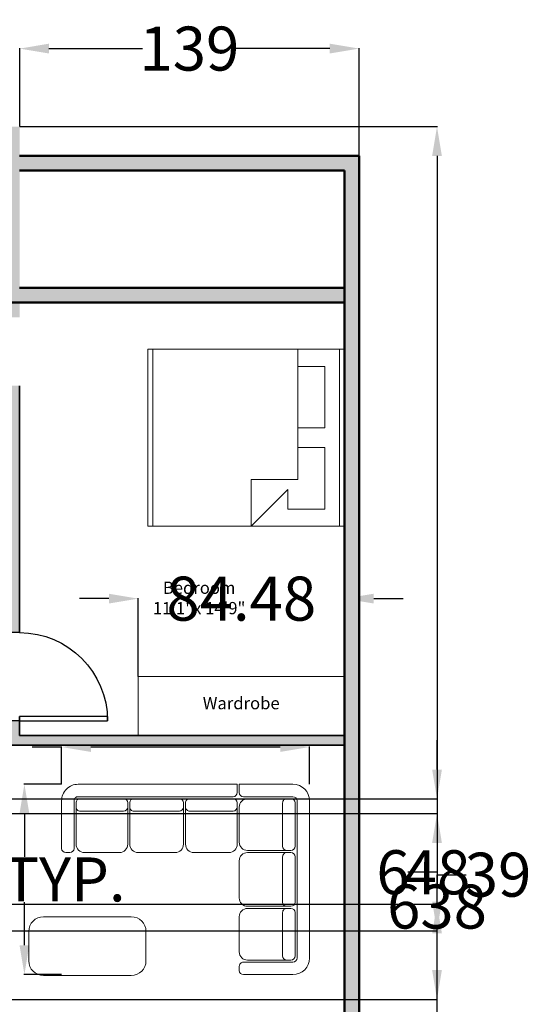
# Model space of a CAD drawing. Units: inches. Extents: x 2 to 695, y -374 to 352.
# Tile 6 of 6: x 421 to 630, y -51 to 352. Entities that reach past the tile are written whole.
import ezdxf

# ---------------------------------------------------------------- set-up
doc = ezdxf.new("R2010")
doc.units = ezdxf.units.IN
for name, color, linetype, lineweight in [('A-ANNO-DIMS', 2, 'Continuous', 18), ('A-ANNO-TEXT', 7, 'Continuous', 18), ('A-AREA-IDEN', 7, 'Continuous', 18), ('A-DOOR', 3, 'Continuous', 25), ('A-WALL-PATT', 252, 'Continuous', 13), ('Furniture', 2, 'Continuous', 18), ('Inner Wall', 5, 'Continuous', 35), ('Outer Wall', 1, 'Continuous', 50)]:
    doc.layers.add(name, color=color, linetype=linetype, lineweight=lineweight)
doc.styles.get("Standard").update_dxf_attribs({"font": 'arial.ttf'})
doc.dimstyles.get("Standard").update_dxf_attribs({"dimtxt": 18, "dimasz": 12, "dimexe": 0.18, "dimexo": 0.0625, "dimgap": 0.09, "dimtad": 0, "dimtih": 1, "dimtoh": 1, "dimdec": 0, "dimzin": 0, "dimdsep": 46, "dimlunit": 3, "dimtxsty": 'Standard', "dimcen": 0.09, "dimadec": 0, "dimazin": 0, "dimtfac": 1, "dimtdec": 0, "dimtofl": 0, "dimtmove": 0, "dimatfit": 3, "dimfxl": 1, "dimtolj": 1, "dimtzin": 0, "dimarcsym": 0})

# ---------------------------------------------------------------- blocks, each defined once
blk = doc.blocks.new('*U2')
for p, q in [((0, 0), (0, -4)), ((36, 0), (36, -4))]:
    blk.add_line(p, q)
blk.add_lwpolyline([(0, 0), (0, 36), (1.75, 36), (1.75, 0)], close=True)
blk.add_arc((0, 0), 36, 0, 90)
blk = doc.blocks.new('A$C2AFA021D')
for p, q in [((0.8, 2.3), (0.2, 2.3)), ((0.2, 2.15), (0.8, 2.15)), ((0.85, 2.2), (0.85, 2.25)), ((0, 2.1), (0, 0.2)), ((0.15, 0.2), (0.15, 2.1)), ((0.175, 1.55), (0.175, 2.075)), ((0.225, 2.125), (0.275, 2.125)), ((0.75, 2.125), (0.275, 2.125)), ((0.325, 2.075), (0.325, 1.55)), ((0.85, 1.6), (0.85, 2.025)), ((0.275, 1.5), (0.225, 1.5)), ((0.225, 1.475), (0.275, 1.475)), ((0.275, 1.5), (0.75, 1.5)), ((0.75, 1.475), (0.275, 1.475)), ((0.175, 0.875), (0.175, 1.425)), ((0.325, 1.425), (0.325, 0.875)), ((0.85, 0.925), (0.85, 1.375)), ((0.175, 0.225), (0.175, 0.75)), ((0.275, 0.825), (0.225, 0.825)), ((0.225, 0.8), (0.275, 0.8)), ((0.275, 0.825), (0.75, 0.825)), ((0.75, 0.8), (0.275, 0.8)), ((0.325, 0.75), (0.325, 0.225)), ((0.875, 0.275), (0.875, 0.725)), ((0.975, 0.825), (1.4, 0.825)), ((1.5, 0.725), (1.5, 0.275)), ((1.525, 0.275), (1.525, 0.725)), ((1.625, 0.825), (2.075, 0.825)), ((2.175, 0.725), (2.175, 0.275)), ((2.2, 0.275), (2.2, 0.725)), ((2.3, 0.825), (2.725, 0.825)), ((2.825, 0.725), (2.825, 0.275)), ((2.85, 0.2), (2.85, 0.775)), ((2.9, 0.825), (2.95, 0.825)), ((3, 0.775), (3, 0.2)), ((0.85, 0.275), (0.85, 0.7)), ((0.875, 0.275), (0.875, 0.225)), ((1.45, 0.325), (0.925, 0.325)), ((1.5, 0.225), (1.5, 0.275)), ((1.525, 0.275), (1.525, 0.225)), ((2.125, 0.325), (1.575, 0.325)), ((2.175, 0.225), (2.175, 0.275)), ((2.2, 0.275), (2.2, 0.225)), ((2.775, 0.325), (2.25, 0.325)), ((2.825, 0.225), (2.825, 0.275)), ((0.8, 0.15), (0.2, 0.15)), ((0.275, 0.175), (0.225, 0.175)), ((0.275, 0.175), (0.75, 0.175)), ((0.925, 0.175), (1.45, 0.175)), ((0.925, 0.15), (2.8, 0.15)), ((1.575, 0.175), (2.125, 0.175)), ((2.25, 0.175), (2.775, 0.175)), ((0.85, 0), (0.85, 0.1)), ((0.875, 0.1), (0.875, 0)), ((0.2, 0), (0.85, 0)), ((2.8, 0), (0.875, 0))]:
    blk.add_line(p, q)
for centre, radius, start, end in [((0.2, 2.1), 0.2, 90, 180), ((0.8, 2.25), 0.05, 0, 90), ((0.2, 2.1), 0.05, 90, 180), ((0.8, 2.2), 0.05, 270, 0), ((0.225, 2.075), 0.05, 90, 180), ((0.275, 2.075), 0.05, 0, 90), ((0.75, 2.025), 0.1, 0, 90), ((0.225, 1.55), 0.05, 180, 270), ((0.275, 1.55), 0.05, 270, 0), ((0.75, 1.6), 0.1, 270, 0), ((0.225, 1.425), 0.05, 90, 180), ((0.275, 1.425), 0.05, 0, 90), ((0.75, 1.375), 0.1, 360, 90), ((0.225, 0.875), 0.05, 180, 270), ((0.275, 0.875), 0.05, 270, 0), ((0.75, 0.925), 0.1, 270, 0), ((0.225, 0.75), 0.05, 90, 180), ((0.275, 0.75), 0.05, 0, 90), ((0.75, 0.7), 0.1, 0, 90), ((0.975, 0.725), 0.1, 90, 180), ((1.4, 0.725), 0.1, 0, 90), ((1.625, 0.725), 0.1, 90, 180), ((2.075, 0.725), 0.1, 0, 90), ((2.3, 0.725), 0.1, 90, 180), ((2.725, 0.725), 0.1, 0, 90), ((2.9, 0.775), 0.05, 90, 180), ((2.95, 0.775), 0.05, 0, 90), ((0.75, 0.275), 0.1, 270, 0), ((0.925, 0.275), 0.05, 90, 180), ((1.45, 0.275), 0.05, 360, 90), ((1.575, 0.275), 0.05, 90, 180), ((2.125, 0.275), 0.05, 360, 90), ((2.25, 0.275), 0.05, 90, 180), ((2.775, 0.275), 0.05, 360, 90), ((0.2, 0.2), 0.2, 180, 270), ((0.2, 0.2), 0.05, 180, 270), ((0.225, 0.225), 0.05, 180, 270), ((0.275, 0.225), 0.05, 270, 0), ((0.8, 0.1), 0.05, 0, 90), ((0.925, 0.225), 0.05, 180, 270), ((0.925, 0.1), 0.05, 90, 180), ((1.45, 0.225), 0.05, 270, 0), ((1.575, 0.225), 0.05, 180, 270), ((2.125, 0.225), 0.05, 270, 0), ((2.25, 0.225), 0.05, 180, 270), ((2.775, 0.225), 0.05, 270, 0), ((2.8, 0.2), 0.2, 270, 0), ((2.8, 0.2), 0.05, 270, 0)]:
    blk.add_arc(centre, radius, start, end)
blk = doc.blocks.new('KING-00')
for p, q in [((-0.897, -0.947), (-0.897, 0.882)), ((0.602, 0.882), (0.602, -0.464)), ((1.034, -0.947), (1.034, 0.882)), ((0.602, 0.704), (0.881, 0.704)), ((0.881, 0.069), (0.881, 0.704)), ((0.602, 0.069), (0.881, 0.069)), ((0.881, -0.134), (0.602, -0.134)), ((0.881, -0.769), (0.881, -0.134)), ((0.119, -0.464), (0.119, -0.947)), ((0.602, -0.464), (0.119, -0.464)), ((0.119, -0.947), (0.5, -0.566)), ((0.5, -0.769), (0.5, -0.566)), ((0.5, -0.769), (0.881, -0.769))]:
    blk.add_line(p, q)
blk.add_lwpolyline([(-0.948, -0.947), (-0.948, 0.882), (1.084, 0.882), (1.084, -0.947)], close=True)
blk = doc.blocks.new('*D18')
at = {"layer": 'A-ANNO-DIMS', "color": 0, "lineweight": -2, "transparency": 16777216}
for p, q in [((437.96, 54.39), (425.96, 54.39)), ((437.96, 39.23), (437.96, 54.57)), ((527.48, 54.39), (449.96, 54.39)), ((539.48, 39.23), (539.48, 54.57))]:
    blk.add_line(p, q, dxfattribs=at)
at = {"layer": 'A-ANNO-DIMS', "color": 0, "transparency": 16777216}
for points in [[(449.96, 56.39), (449.96, 52.39), (437.96, 54.39)], [(527.48, 56.39), (527.48, 52.39), (539.48, 54.39)]]:
    blk.add_solid(points, dxfattribs=at)
at = {"layer": 'Defpoints', "color": 0, "transparency": 16777216}
for p in [(437.96, 54.39), (437.96, 39.17), (539.48, 39.17)]:
    blk.add_point(p, dxfattribs=at)
at = {"layer": 'A-ANNO-DIMS', "color": 0, "transparency": 16777216, "insert": (337.39, 54.39), "char_height": 18, "attachment_point": 5}
blk.add_mtext('\\A1;SOFA 102 TYP.', dxfattribs=at)
blk = doc.blocks.new('*D19')
at = {"layer": 'A-ANNO-DIMS', "color": 0, "lineweight": -2, "transparency": 16777216}
for p, q in [((437.9, 39.17), (422.55, 39.17)), ((422.73, 27.17), (422.73, 9.53)), ((422.73, -26.67), (422.73, -9.03)), ((437.9, -38.67), (422.55, -38.67))]:
    blk.add_line(p, q, dxfattribs=at)
at = {"layer": 'A-ANNO-DIMS', "color": 0, "transparency": 16777216}
for points in [[(420.73, 27.17), (424.73, 27.17), (422.73, 39.17)], [(420.73, -26.67), (424.73, -26.67), (422.73, -38.67)]]:
    blk.add_solid(points, dxfattribs=at)
at = {"layer": 'Defpoints', "color": 0, "transparency": 16777216}
for p in [(437.96, 39.17), (422.73, -38.67), (437.96, -38.67)]:
    blk.add_point(p, dxfattribs=at)
at = {"layer": 'A-ANNO-DIMS', "color": 0, "transparency": 16777216, "insert": (422.73, 0.25), "char_height": 18, "attachment_point": 5}
blk.add_mtext('\\A1;78 TYP.', dxfattribs=at)
blk = doc.blocks.new('*D29')
at = {"layer": 'A-ANNO-DIMS', "color": 0, "lineweight": -2, "transparency": 16777216}
for p, q in [((420.85, 308.13), (591.88, 308.13)), ((591.7, 296.13), (591.7, -1.56)), ((591.7, -317.82), (591.7, -20.13)), ((217.35, -329.82), (591.88, -329.82))]:
    blk.add_line(p, q, dxfattribs=at)
at = {"layer": 'A-ANNO-DIMS', "color": 0, "transparency": 16777216}
for points in [[(589.7, 296.13), (593.7, 296.13), (591.7, 308.13)], [(589.7, -317.82), (593.7, -317.82), (591.7, -329.82)]]:
    blk.add_solid(points, dxfattribs=at)
at = {"layer": 'Defpoints', "color": 0, "transparency": 16777216}
for p in [(420.79, 308.13), (591.7, 308.13), (217.29, -329.82)]:
    blk.add_point(p, dxfattribs=at)
at = {"layer": 'A-ANNO-DIMS', "color": 0, "transparency": 16777216, "insert": (591.7, -10.85), "char_height": 18, "attachment_point": 5}
blk.add_mtext('\\A1;638', dxfattribs=at)
blk = doc.blocks.new('*D32')
at = {"layer": 'A-ANNO-DIMS', "color": 0, "lineweight": -2, "transparency": 16777216}
for p, q in [((420.79, 308.19), (420.79, 340.22)), ((432.79, 340.04), (471.14, 340.04)), ((547.79, 340.04), (509.43, 340.04)), ((559.79, 296.24), (559.79, 340.22))]:
    blk.add_line(p, q, dxfattribs=at)
at = {"layer": 'A-ANNO-DIMS', "color": 0, "transparency": 16777216}
for points in [[(432.79, 342.04), (432.79, 338.04), (420.79, 340.04)], [(547.79, 342.04), (547.79, 338.04), (559.79, 340.04)]]:
    blk.add_solid(points, dxfattribs=at)
at = {"layer": 'Defpoints', "color": 0, "transparency": 16777216}
for p in [(559.79, 340.04), (420.79, 308.13), (559.79, 296.18)]:
    blk.add_point(p, dxfattribs=at)
at = {"layer": 'A-ANNO-DIMS', "color": 0, "transparency": 16777216, "insert": (490.29, 340.04), "char_height": 18, "attachment_point": 5}
blk.add_mtext('\\A1;139', dxfattribs=at)
blk = doc.blocks.new('*D38')
at = {"layer": 'A-ANNO-DIMS', "color": 0, "lineweight": -2, "transparency": 16777216}
for p, q in [((350.85, 27.18), (591.88, 27.18)), ((591.7, 15.18), (591.7, 12.46)), ((591.7, -8.82), (591.7, -6.11)), ((350.85, -20.82), (591.88, -20.82))]:
    blk.add_line(p, q, dxfattribs=at)
at = {"layer": 'A-ANNO-DIMS', "color": 0, "transparency": 16777216}
for points in [[(589.7, 15.18), (593.7, 15.18), (591.7, 27.18)], [(589.7, -8.82), (593.7, -8.82), (591.7, -20.82)]]:
    blk.add_solid(points, dxfattribs=at)
at = {"layer": 'Defpoints', "color": 0, "transparency": 16777216}
for p in [(350.79, 27.18), (350.79, -20.82), (591.7, -20.82)]:
    blk.add_point(p, dxfattribs=at)
at = {"layer": 'A-ANNO-DIMS', "color": 0, "transparency": 16777216, "insert": (591.7, 3.18), "char_height": 18, "attachment_point": 5}
blk.add_mtext('\\A1;48', dxfattribs=at)
blk = doc.blocks.new('*D49')
at = {"layer": 'A-ANNO-DIMS', "color": 0, "lineweight": -2, "transparency": 16777216}
for p, q in [((591.7, -9.82), (591.7, 2.18)), ((591.7, 2.18), (603.7, 2.18)), ((291.85, -9.82), (591.88, -9.82)), ((591.7, -36.82), (591.7, -21.82)), ((291.85, -48.82), (591.88, -48.82))]:
    blk.add_line(p, q, dxfattribs=at)
at = {"layer": 'A-ANNO-DIMS', "color": 0, "transparency": 16777216}
for points in [[(589.7, -21.82), (593.7, -21.82), (591.7, -9.82)], [(589.7, -36.82), (593.7, -36.82), (591.7, -48.82)]]:
    blk.add_solid(points, dxfattribs=at)
at = {"layer": 'Defpoints', "color": 0, "transparency": 16777216}
for p in [(291.79, -9.82), (591.7, -9.82), (291.79, -48.82)]:
    blk.add_point(p, dxfattribs=at)
at = {"layer": 'A-ANNO-DIMS', "color": 0, "transparency": 16777216, "insert": (616.7, 2.18), "char_height": 18, "attachment_point": 5}
blk.add_mtext('\\A1;39', dxfattribs=at)
blk = doc.blocks.new('*D50')
at = {"layer": 'A-ANNO-DIMS', "color": 0, "lineweight": -2, "transparency": 16777216}
for p, q in [((591.7, 45.18), (591.7, 57.18)), ((346.85, 33.18), (591.88, 33.18)), ((346.85, 27.18), (591.88, 27.18)), ((591.7, 15.18), (591.7, 3.18)), ((591.7, 3.18), (579.7, 3.18))]:
    blk.add_line(p, q, dxfattribs=at)
at = {"layer": 'A-ANNO-DIMS', "color": 0, "transparency": 16777216}
for points in [[(589.7, 45.18), (593.7, 45.18), (591.7, 33.18)], [(589.7, 15.18), (593.7, 15.18), (591.7, 27.18)]]:
    blk.add_solid(points, dxfattribs=at)
at = {"layer": 'Defpoints', "color": 0, "transparency": 16777216}
for p in [(346.79, 33.18), (346.79, 27.18), (591.7, 27.18)]:
    blk.add_point(p, dxfattribs=at)
at = {"layer": 'A-ANNO-DIMS', "color": 0, "transparency": 16777216, "insert": (573.67, 3.18), "char_height": 18, "attachment_point": 5}
blk.add_mtext('\\A1;6', dxfattribs=at)
blk = doc.blocks.new('*D52')
at = {"layer": 'A-ANNO-DIMS', "color": 0, "lineweight": -2, "transparency": 16777216}
for p, q in [((457.307121, 115.090046), (445.307121, 115.090046)), ((469.307121, 83.237546), (469.307121, 115.270046)), ((553.785845, 83.237546), (553.785845, 115.270046)), ((565.785845, 115.090046), (577.785845, 115.090046))]:
    blk.add_line(p, q, dxfattribs=at)
at = {"layer": 'A-ANNO-DIMS', "color": 0, "transparency": 16777216}
for points in [[(457.307121, 117.090046), (457.307121, 113.090046), (469.307121, 115.090046)], [(565.785845, 117.090046), (565.785845, 113.090046), (553.785845, 115.090046)]]:
    blk.add_solid(points, dxfattribs=at)
at = {"layer": 'Defpoints', "color": 0, "transparency": 16777216}
for p in [(553.785845, 115.090046), (469.307121, 83.175046), (553.785845, 83.175046)]:
    blk.add_point(p, dxfattribs=at)
at = {"layer": 'A-ANNO-DIMS', "color": 0, "transparency": 16777216, "insert": (511.546483, 115.090046), "char_height": 18, "attachment_point": 5}
blk.add_mtext('\\A1;84.48', dxfattribs=at)

msp = doc.modelspace()

# ---------------------------------------------------------------- hatches: boundary and pattern name
at = {"layer": 'A-WALL-PATT'}
h = msp.add_hatch(color=256, dxfattribs=at)
h.dxf.hatch_style = 1
h.paths.add_polyline_path([(346.7858, 296.175), (146.7858, 296.175), (146.7858, -329.825), (217.2858, -329.825), (217.2858, -305.825), (559.7858, -305.825), (559.7858, 296.175), (420.7858, 296.175), (420.7858, 290.175), (553.7858, 290.175), (553.7858, -299.825), (213.2858, -299.825), (213.2858, -323.825), (152.7858, -323.825), (152.7858, 290.175), (346.7858, 290.175)])
h.paths.add_polyline_path([(420.7858, 308.1298), (346.7858, 308.1298), (346.7858, 242.175), (228.7858, 242.175), (228.7858, 264.175), (152.7858, 264.175), (152.7858, 260.175), (224.7858, 260.175), (224.7858, 236.175), (350.7858, 236.175), (350.7858, 302.1298), (416.7858, 302.1298), (416.7858, 236.175), (553.7858, 236.175), (553.7858, 242.175), (420.7858, 242.175)])
h = msp.add_hatch(color=256, dxfattribs=at)
h.dxf.hatch_style = 1
h.paths.add_polyline_path([(394.2858, -160.825), (390.2858, -160.825), (390.2858, -164.825), (390.2858, -299.825), (394.2858, -299.825)])
h.paths.add_polyline_path([(217.2858, -235.1253), (213.2858, -235.1253), (213.2858, -299.825), (217.2858, -299.825)])
h.paths.add_polyline_path([(213.2858, -273.825), (152.7858, -273.825), (152.7858, -275.825), (213.2858, -275.825)])
h.paths.add_polyline_path([(354.2858, -160.825), (350.7858, -160.825), (350.7858, -124.825), (346.7858, -124.825), (346.7858, -160.825), (152.7858, -160.825), (152.7858, -164.825), (213.2858, -164.825), (213.2858, -188.8137), (213.2858, -207.1253), (217.2858, -207.1253), (217.2858, -187.1253), (217.2858, -164.825), (354.2858, -164.825)])
h.paths.add_polyline_path([(350.7858, -20.825), (346.7858, -20.825), (346.7858, -48.825), (152.7858, -48.825), (152.7858, -52.825), (249.7858, -52.825), (346.7858, -52.825), (346.7858, -88.825), (350.7858, -88.825)])
h.paths.add_polyline_path([(189.7858, 33.175), (185.7858, 33.175), (185.7858, -48.825), (189.7858, -48.825)])
h.paths.add_polyline_path([(334.7858, 37.175), (264.7858, 37.175), (264.7858, 33.175), (334.7858, 33.175)])
h.paths.add_polyline_path([(258.7858, 37.175), (152.7858, 37.175), (152.7858, 33.175), (258.7858, 33.175)])
h.paths.add_polyline_path([(194.7858, 101.175), (192.7858, 101.175), (192.7858, 37.175), (194.7858, 37.175)])
h.paths.add_polyline_path([(264.7858, 105.175), (258.7858, 105.175), (258.7858, 33.175), (264.7858, 33.175), (264.7858, 37.175)])
h.paths.add_polyline_path([(340.7858, 105.175), (334.7858, 105.175), (334.7858, 33.175), (340.7858, 33.175)])
h.paths.add_polyline_path([(350.7858, 111.175), (346.7858, 111.175), (346.7858, 105.175), (340.7858, 105.175), (340.7858, 101.175), (350.7858, 101.175)])
h.paths.add_polyline_path([(350.7858, 37.175), (340.7858, 37.175), (340.7858, 33.175), (346.7858, 33.175), (346.7858, 27.175), (350.7858, 27.175)])
h.paths.add_polyline_path([(334.7858, 105.175), (264.7858, 105.175), (264.7858, 101.175), (334.7858, 101.175)])
h.paths.add_polyline_path([(258.7858, 105.175), (252.7858, 105.175), (252.7858, 101.175), (258.7858, 101.175)])
h.paths.add_polyline_path([(224.7858, 105.175), (152.7858, 105.175), (152.7858, 101.175), (224.7858, 101.175)])
h.paths.add_polyline_path([(382.7858, 165.1298), (350.7858, 165.1298), (350.7858, 161.1298), (382.7858, 161.1298)])
h.paths.add_polyline_path([(350.7858, 236.175), (346.7858, 236.175), (346.7858, 147.175), (350.7858, 147.175)])
h.paths.add_polyline_path([(420.7858, 202.175), (416.7858, 202.175), (416.7858, 101.175), (420.7858, 101.175)])
h.paths.add_polyline_path([(416.7858, 165.1298), (410.7858, 165.1298), (410.7858, 161.1298), (416.7858, 161.1298)])
h.paths.add_polyline_path([(416.7858, 242.175), (350.7858, 242.175), (350.7858, 240.175), (416.7858, 240.175)])
h.paths.add_polyline_path([(420.7858, 236.175), (416.7858, 236.175), (416.7858, 230.175), (420.7858, 230.175)])
h.paths.add_polyline_path([(553.7858, 59.175), (469.3071, 59.175), (420.7858, 59.175), (420.7858, 65.175), (416.7858, 65.175), (416.7858, 55.175), (553.7858, 55.175)])

# ---------------------------------------------------------------- linework, layer by layer
at = {"layer": 'Furniture'}
msp.add_lwpolyline([(469.3071, 83.175), (553.7858, 83.175), (553.7858, 59.175), (469.3071, 59.175)], close=True, dxfattribs=at)
msp.add_lwpolyline([(424.5089, -33.0365), (424.5089, -21.0365, -0.41421356), (430.5089, -15.0365), (466.5089, -15.0365, -0.41421356), (472.5089, -21.0365), (472.5089, -33.0365, -0.41421356), (466.5089, -39.0365), (430.5089, -39.0365, -0.41421356)], format="xyb", close=True, dxfattribs=at)
at = {"layer": 'Inner Wall'}
for p, q in [((420.7858, 101.175), (420.7858, 202.175)), ((420.7858, 59.175), (420.7858, 66.925)), ((420.7858, 59.175), (553.7858, 59.175)), ((416.7858, 55.175), (553.7858, 55.175))]:
    msp.add_line(p, q, dxfattribs=at)
at = {"layer": 'Outer Wall'}
for p, q in [((559.7858, 296.175), (420.7858, 296.175)), ((559.7858, -305.825), (559.7858, 296.175)), ((553.7858, 290.175), (420.7858, 290.175)), ((553.7858, -299.825), (553.7858, 290.175)), ((420.7858, 242.175), (553.7858, 242.175)), ((416.7858, 236.175), (553.7858, 236.175))]:
    msp.add_line(p, q, dxfattribs=at)

# ---------------------------------------------------------------- block references
at = {"layer": 'A-DOOR', "xscale": -1, "rotation": 270}
msp.add_blockref('*U2', (420.7858, 65.175), dxfattribs=at)
at = {"layer": 'Furniture', "xscale": 39.60249106241186, "yscale": 39.60249106241186, "zscale": 39.60249106241186}
msp.add_blockref('KING-00', (510.837, 182.1583), dxfattribs=at)
at = {"layer": 'Furniture', "xscale": 33.84012530478223, "yscale": 33.84012530478223, "zscale": 33.84012530478223, "rotation": 180}
msp.add_blockref('A$C2AFA021D', (539.4825, 39.1654), dxfattribs=at)

# ---------------------------------------------------------------- texts
at = {"layer": 'A-ANNO-TEXT', "insert": (536.0715, 74.8333), "char_height": 5, "attachment_point": 3}
msp.add_mtext_dynamic_manual_height_columns('\\pxqc;{\\fTimes New Roman|b0|i0|c0|p18;Wardrobe}', width=49.101878, gutter_width=12.5, heights=[0], dxfattribs=at)
at = {"layer": 'A-AREA-IDEN', "insert": (518.8254, 122.0309), "char_height": 5, "attachment_point": 3}
msp.add_mtext_dynamic_manual_height_columns('\\pxqc;{\\fTimes New Roman|b0|i0|c0|p18;Bedroom\\P11\'1"x 14\'9"}', width=49.101878, gutter_width=12.5, heights=[0], dxfattribs=at)

# ---------------------------------------------------------------- dimensions: what is measured, and where the dimension line sits
at = {"layer": 'A-ANNO-DIMS'}
for base, p1, p2, override, picture, middle in [((559.7858, 340.0448), (420.7858, 308.1298), (559.7858, 296.175), {"dimdec": 0, "dimlfac": 1, "dimrnd": 0, "dimzin": 0, "dimdsep": 46, "dimlunit": 2}, '*D32', (490.2858, 340.0448)), ((553.7858, 115.09), (469.3071, 83.175), (553.7858, 83.175), {"dimdec": 2, "dimlfac": 1, "dimrnd": 0, "dimzin": 0, "dimdsep": 46, "dimlunit": 2}, '*D52', (511.5465, 115.09))]:
    dim = msp.add_linear_dim(base=base, p1=p1, p2=p2, dimstyle='Standard', override=override, dxfattribs=at)
    dim.commit()
    dim.dimension.update_dxf_attribs({"geometry": picture, "text_midpoint": middle})
for base, p1, p2, picture, middle in [((591.7008, 308.1298), (217.2858, -329.825), (420.7858, 308.1298), '*D29', (591.7008, -10.8476)), ((591.7008, 27.175), (346.7858, 33.175), (346.7858, 27.175), '*D50', (573.6681, 3.175)), ((591.7008, -20.825), (350.7858, 27.175), (350.7858, -20.825), '*D38', (591.7008, 3.175)), ((591.7008, -9.825), (291.7858, -48.825), (291.7858, -9.825), '*D49', (616.6953, 2.175))]:
    dim = msp.add_linear_dim(base=base, p1=p1, p2=p2, angle=90, dimstyle='Standard', override={"dimdec": 0, "dimlfac": 1, "dimrnd": 0, "dimzin": 0, "dimdsep": 46, "dimlunit": 2}, dxfattribs=at)
    dim.commit()
    dim.dimension.update_dxf_attribs({"geometry": picture, "text_midpoint": middle})
for base, p1, p2, angle, text, picture, middle in [((437.9621, 54.3935), (539.4825, 39.1654), (437.9621, 39.1654), 180, 'SOFA <> TYP.', '*D18', (337.3885, 54.3935)), ((422.7341, -38.6669), (437.9621, 39.1654), (437.9621, -38.6669), 270, '<> TYP.', '*D19', (422.7341, 0.2493))]:
    dim = msp.add_linear_dim(base=base, p1=p1, p2=p2, angle=angle, text=text, dimstyle='Standard', override={"dimdec": 0, "dimlfac": 1, "dimrnd": 0, "dimzin": 0, "dimdsep": 46, "dimlunit": 2}, dxfattribs=at)
    dim.commit()
    dim.dimension.update_dxf_attribs({"geometry": picture, "text_midpoint": middle})

doc.saveas('drawing.dxf')
